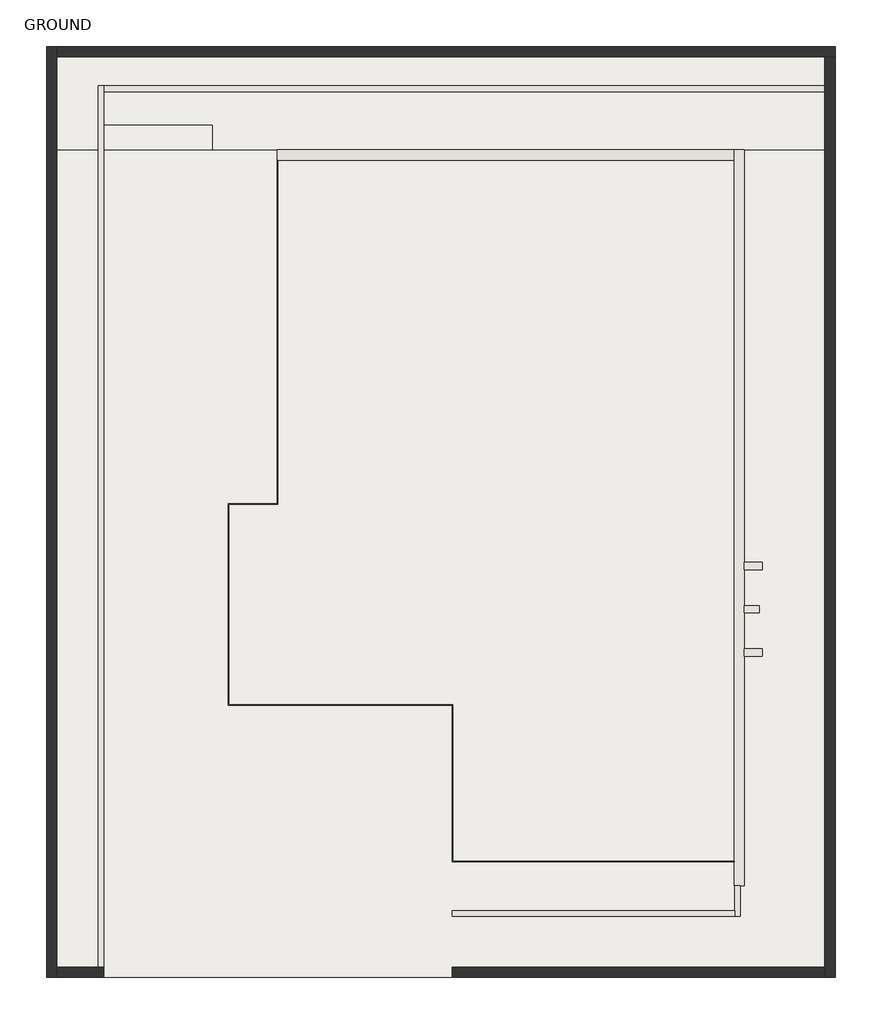
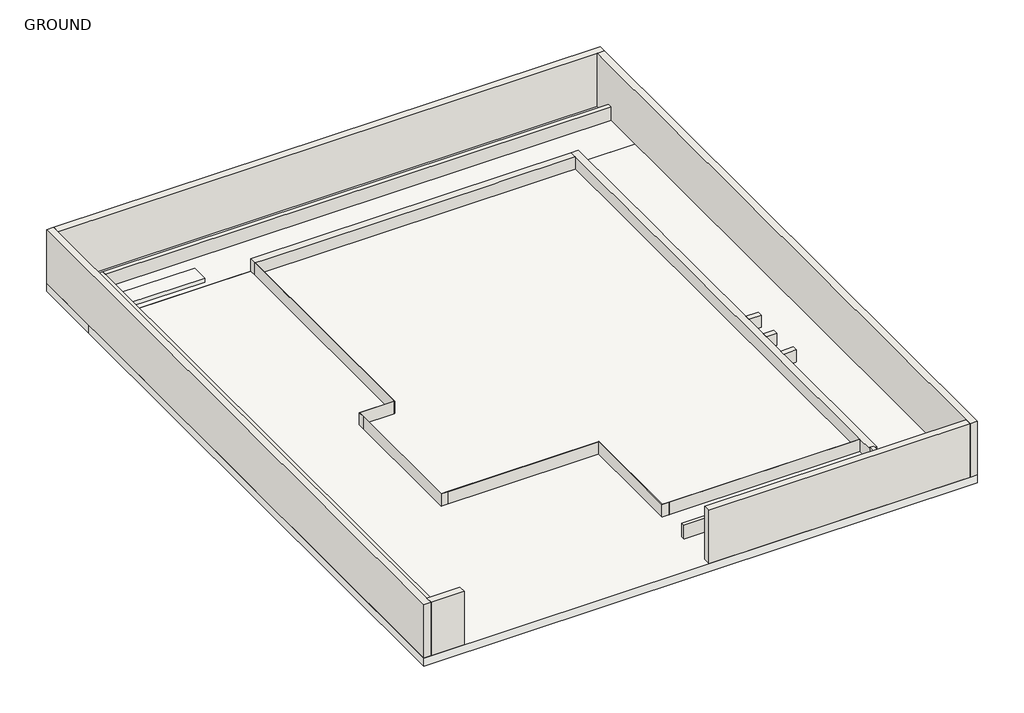
# One storey: 20 walls, 3 slabs.
"""IFC4 building model written with IfcOpenShell, lengths in millimetres."""

from ifc_helpers import new_model, si_unit, frame, origin, origin_with_axes, place, context, project, spatial, polyline, outline, extrude, faceted_brep, element, save

model = new_model("IFC4")

# Units and contexts
model_context = context("Model", 3, world=origin())
ifc_project = project(units=[si_unit("LENGTHUNIT", "METRE", prefix="MILLI")], contexts=[model_context])

# Site, building, storey
site = spatial("IfcSite", under=ifc_project)
building = spatial("IfcBuilding", under=site)
storey = spatial("IfcBuildingStorey", under=building, Name="GROUND", Elevation=0.0)

# Slabs
placement = place(None, origin())
element("IfcSlab", 1, ObjectType="6\" 3", at=placement, inside=storey, context=model_context, shape_type="SweptSolid", body=[
    extrude(outline(polyline([(-6900.6561363, 9478.9935985), (-9643.8561363, 9478.9935985), (-9643.8561363, 10088.5935985), (-6900.6561363, 10088.5935985), (-6900.6561363, 9478.9935985)])), frame((0.0, 0.0, 152.4), z_axis=(0.0, 0.0, 1.0), x_axis=(1.0, 0.0, 0.0)), (0.0, 0.0, 1.0), 152.4),
])
element("IfcSlab", 2, ObjectType="Generic - 12\"", at=placement, inside=storey, context=model_context, shape_type="SweptSolid", body=[
    extrude(outline(polyline([(8479.5731195, 9466.0221373), (8479.5731195, -10955.3064015), (-10990.0561363, -10955.3064015), (-10990.0561363, 9466.0221373), (8479.5731195, 9466.0221373)])), frame((0.0, 0.0, -304.8), z_axis=(0.0, 0.0, 1.0), x_axis=(1.0, 0.0, 0.0)), (0.0, 0.0, 1.0), 304.8),
])
element("IfcSlab", 3, ObjectType="Generic - 12\" 2", at=placement, inside=storey, context=model_context, shape_type="SweptSolid", body=[
    extrude(outline(polyline([(8479.5731195, 12031.6935985), (8479.5731195, 9466.0221373), (-10990.0561363, 9466.0221373), (-10990.0561363, 12031.6935985), (8479.5731195, 12031.6935985)])), frame((0.0, 0.0, -304.8), z_axis=(0.0, 0.0, 1.0), x_axis=(1.0, 0.0, 0.0)), (0.0, 0.0, 1.0), 304.8),
])

# Walls
element("IfcWall", 4, ObjectType="4.5\"", at=placement, inside=storey, context=model_context, shape_type="Brep", body=[
    faceted_brep([(-9574.0061363, -10701.3064015, 0.0), (-9574.0061363, 10920.4435985, 0.0), (-9574.0061363, 11060.1435985, 0.0), (-9574.0061363, 11060.1435985, 508.0), (-9574.0061363, 10920.4435985, 508.0), (-9574.0061363, -10701.3064015, 508.0), (-9713.7061363, -10701.3064015, 0.0), (-9713.7061363, -10701.3064015, 508.0), (-9713.7061363, 11060.1435985, 508.0), (-9713.7061363, 11060.1435985, 0.0)], [[[0, 1, 2, 3, 4, 5]], [[6, 7, 8, 9]], [[2, 1, 0, 6, 9]], [[5, 4, 3, 8, 7]], [[3, 2, 9, 8]], [[0, 5, 7, 6]]]),
])
element("IfcWall", 5, ObjectType="4.5\"", at=placement, inside=storey, context=model_context, shape_type="SweptSolid", body=[
    extrude(outline(polyline([(8225.5731195, 10920.4435985), (-9574.0061363, 10920.4435985), (-9574.0061363, 11060.1435985), (8225.5731195, 11060.1435985), (8225.5731195, 10920.4435985)])), origin_with_axes(), (0.0, 0.0, 1.0), 508.0),
])
element("IfcWall", 6, ObjectType="4.5\"", at=placement, inside=storey, context=model_context, shape_type="Brep", body=[
    faceted_brep([(6002.8084916, -8694.7064015, 508.0), (6002.8084916, -8694.7064015, 0.0), (6002.8084916, -9304.3064015, 0.0), (6002.8084916, -9444.0064015, 0.0), (6002.8084916, -9444.0064015, 508.0), (6002.8084916, -9304.3064015, 508.0), (6142.5084916, -8694.7064015, 0.0), (6142.5084916, -8694.7064015, 508.0), (6142.5084916, -9444.0064015, 508.0), (6142.5084916, -9444.0064015, 0.0)], [[[0, 1, 2, 3, 4, 5]], [[6, 7, 8, 9]], [[3, 2, 1, 6, 9]], [[0, 5, 4, 8, 7]], [[4, 3, 9, 8]], [[0, 7, 6, 1]]]),
])
element("IfcWall", 7, ObjectType="4.5\"", at=placement, inside=storey, context=model_context, shape_type="SweptSolid", body=[
    extrude(outline(polyline([(-969.7561363, -9304.3064015), (6002.8084916, -9304.3064015), (6002.8084916, -9444.0064015), (-969.7561363, -9444.0064015), (-969.7561363, -9304.3064015)])), origin_with_axes(), (0.0, 0.0, 1.0), 508.0),
])
element("IfcWall", 8, ObjectType="6\" WALL", at=placement, inside=storey, context=model_context, shape_type="SweptSolid", body=[
    extrude(outline(polyline([(6688.3438637, -885.2318739), (6244.1084916, -885.2318739), (6244.1084916, -707.4318739), (6688.3438637, -707.4318739), (6688.3438637, -885.2318739)])), origin_with_axes(), (0.0, 0.0, 1.0), 457.2),
])
element("IfcWall", 9, ObjectType="6\" WALL", at=placement, inside=storey, context=model_context, shape_type="SweptSolid", body=[
    extrude(outline(polyline([(6244.1084916, -2840.9358398), (6688.3438637, -2840.9358398), (6688.3438637, -3018.7358398), (6244.1084916, -3018.7358398), (6244.1084916, -2840.9358398)])), origin_with_axes(), (0.0, 0.0, 1.0), 457.2),
])
element("IfcWall", 10, ObjectType="6\" WALL", at=placement, inside=storey, context=model_context, shape_type="SweptSolid", body=[
    extrude(outline(polyline([(6244.1084916, -1774.2318739), (6612.1438637, -1774.2318739), (6612.1438637, -1952.0318739), (6244.1084916, -1952.0318739), (6244.1084916, -1774.2318739)])), origin_with_axes(), (0.0, 0.0, 1.0), 457.2),
])
element("IfcWall", 11, ObjectType="9\"", at=placement, inside=storey, context=model_context, shape_type="SweptSolid", body=[
    extrude(outline(polyline([(5990.1084916, -8097.8064015), (-715.7561363, -8097.8064015), (-715.7561363, -8085.3778627), (5990.1084916, -8085.3778627), (5990.1084916, -8097.8064015)])), origin_with_axes(), (0.0, 0.0, 1.0), 457.2),
])
element("IfcWall", 12, ObjectType="9\"", at=placement, inside=storey, context=model_context, shape_type="Brep", body=[
    faceted_brep([(5990.1084916, 9478.9935985, 0.0), (5990.1084916, 9224.9935985, 0.0), (5990.1084916, -8085.3778627, 0.0), (5990.1084916, -8097.8064015, 0.0), (5990.1084916, -8694.7064015, 0.0), (5990.1084916, -8694.7064015, 457.2), (5990.1084916, -8097.8064015, 457.2), (5990.1084916, -8085.3778627, 457.2), (5990.1084916, 1978.0935985, 457.2), (5990.1084916, 2943.2935985, 457.2), (5990.1084916, 3938.6935985, 457.2), (5990.1084916, 4751.4935985, 457.2), (5990.1084916, 9224.9935985, 457.2), (5990.1084916, 9478.9935985, 457.2), (6244.1084916, 9478.9935985, 0.0), (6244.1084916, 9478.9935985, 457.2), (6244.1084916, 4751.4935985, 457.2), (6244.1084916, 3938.6935985, 457.2), (6244.1084916, 2943.2935985, 457.2), (6244.1084916, 1978.0935985, 457.2), (6244.1084916, -707.4318739, 457.2), (6244.1084916, -885.2318739, 457.2), (6244.1084916, -1774.2318739, 457.2), (6244.1084916, -1952.0318739, 457.2), (6244.1084916, -2840.9358398, 457.2), (6244.1084916, -3018.7358398, 457.2), (6244.1084916, -8694.7064015, 457.2), (6244.1084916, -8694.7064015, 0.0), (6244.1084916, -3018.7358398, 0.0), (6244.1084916, -2840.9358398, 0.0), (6244.1084916, -1952.0318739, 0.0), (6244.1084916, -1774.2318739, 0.0), (6244.1084916, -885.2318739, 0.0), (6244.1084916, -707.4318739, 0.0), (6142.5084916, -8694.7064015, 0.0), (6002.8084916, -8694.7064015, 0.0)], [[[0, 1, 2, 3, 4, 5, 6, 7, 8, 9, 10, 11, 12, 13]], [[14, 15, 16, 17, 18, 19, 20, 21, 22, 23, 24, 25, 26, 27, 28, 29, 30, 31, 32, 33]], [[4, 3, 2, 1, 0, 14, 33, 32, 31, 30, 29, 28, 27, 34, 35]], [[5, 4, 35, 34, 27, 26]], [[13, 12, 11, 10, 9, 8, 7, 6, 5, 26, 25, 24, 23, 22, 21, 20, 19, 18, 17, 16, 15]], [[0, 13, 15, 14]]]),
])
element("IfcWall", 13, ObjectType="9\"", at=placement, inside=storey, context=model_context, shape_type="Brep", body=[
    faceted_brep([(5990.1084916, 9478.9935985, 0.0), (-5287.7561363, 9478.9935985, 0.0), (-5287.7561363, 9478.9935985, 457.2), (5990.1084916, 9478.9935985, 457.2), (5990.1084916, 9224.9935985, 0.0), (5990.1084916, 9224.9935985, 457.2), (3322.8438637, 9224.9935985, 457.2), (3145.0438637, 9224.9935985, 457.2), (-5033.7561363, 9224.9935985, 457.2), (-5287.7561363, 9224.9935985, 457.2), (-5287.7561363, 9224.9935985, 0.0), (-5033.7561363, 9224.9935985, 0.0), (3145.0438637, 9224.9935985, 0.0), (3322.8438637, 9224.9935985, 0.0)], [[[0, 1, 2, 3]], [[4, 5, 6, 7, 8, 9, 10, 11, 12, 13]], [[1, 0, 4, 13, 12, 11, 10]], [[3, 2, 9, 8, 7, 6, 5]], [[0, 3, 5, 4]], [[2, 1, 10, 9]]]),
])
element("IfcWall", 14, ObjectType="9\"", at=placement, inside=storey, context=model_context, shape_type="Brep", body=[
    faceted_brep([(-5287.7561363, 9224.9935985, 457.2), (-5287.7561363, 9224.9935985, 0.0), (-5287.7561363, 741.1221373, 0.0), (-5287.7561363, 728.4221373, 0.0), (-5287.7561363, 728.4221373, 457.2), (-5287.7561363, 741.1221373, 457.2), (-5275.0561363, 9224.9935985, 0.0), (-5275.0561363, 728.4221373, 0.0), (-5275.0561363, 728.4221373, 457.2), (-5275.0561363, 9224.9935985, 457.2)], [[[0, 1, 2, 3, 4, 5]], [[3, 2, 1, 6, 7]], [[0, 5, 4, 8, 9]], [[1, 0, 9, 6]], [[7, 8, 4, 3]], [[8, 7, 6, 9]]]),
])
element("IfcWall", 15, ObjectType="9\"", at=placement, inside=storey, context=model_context, shape_type="SweptSolid", body=[
    extrude(outline(polyline([(-6507.1004467, 741.1221373), (-5287.7561363, 741.1221373), (-5287.7561363, 728.4221373), (-6494.2561363, 728.4221373), (-6494.2561363, 487.1221373), (-6507.1004467, 487.1221373), (-6507.1004467, 741.1221373)])), origin_with_axes(), (0.0, 0.0, 1.0), 457.2),
])
element("IfcWall", 16, ObjectType="9\"", at=placement, inside=storey, context=model_context, shape_type="SweptSolid", body=[
    extrude(outline(polyline([(-6507.1004467, -4237.1266767), (-6507.1004467, 487.1221373), (-6494.2561363, 487.1221373), (-6494.2561363, -4224.5778627), (-6253.1004467, -4224.5778627), (-6253.1004467, -4237.1266767), (-6507.1004467, -4237.1266767)])), origin_with_axes(), (0.0, 0.0, 1.0), 457.2),
])
element("IfcWall", 17, ObjectType="9\"", at=placement, inside=storey, context=model_context, shape_type="SweptSolid", body=[
    extrude(outline(polyline([(-969.7561363, -4237.1266767), (-6253.1004467, -4237.1266767), (-6253.1004467, -4224.5778627), (-969.7561363, -4224.5778627), (-969.7561363, -4237.1266767)])), origin_with_axes(), (0.0, 0.0, 1.0), 457.2),
])
element("IfcWall", 18, ObjectType="9\"", at=placement, inside=storey, context=model_context, shape_type="Brep", body=[
    faceted_brep([(-715.7561363, -8097.8064015, 457.2), (-715.7561363, -8097.8064015, 0.0), (-715.7561363, -8085.3778627, 0.0), (-715.7561363, -8085.3778627, 457.2), (-969.7561363, -8097.8064015, 0.0), (-969.7561363, -8097.8064015, 457.2), (-969.7561363, -4237.1266767, 457.2), (-969.7561363, -4224.5778627, 457.2), (-969.7561363, -4224.5778627, 0.0), (-969.7561363, -4237.1266767, 0.0), (-957.0561363, -4224.5778627, 0.0), (-957.0561363, -8085.3778627, 0.0), (-957.0561363, -8085.3778627, 457.2), (-957.0561363, -4224.5778627, 457.2)], [[[0, 1, 2, 3]], [[4, 5, 6, 7, 8, 9]], [[1, 4, 9, 8, 10, 11, 2]], [[5, 0, 3, 12, 13, 7, 6]], [[1, 0, 5, 4]], [[11, 12, 3, 2]], [[12, 11, 10, 13]], [[13, 10, 8, 7]]]),
])
element("IfcWall", 19, ObjectType="9\"", at=placement, inside=storey, context=model_context, shape_type="Brep", body=[
    faceted_brep([(-10736.0561363, -10955.3064015, 0.0), (-10736.0561363, -10701.3064015, 0.0), (-10736.0561363, 11777.6935985, 0.0), (-10736.0561363, 12031.6935985, 0.0), (-10736.0561363, 12031.6935985, 1981.2), (-10736.0561363, 11777.6935985, 1981.2), (-10736.0561363, -10701.3064015, 1981.2), (-10736.0561363, -10955.3064015, 1981.2), (-10990.0561363, -10955.3064015, 0.0), (-10990.0561363, -10955.3064015, 1981.2), (-10990.0561363, 12031.6935985, 1981.2), (-10990.0561363, 12031.6935985, 0.0)], [[[0, 1, 2, 3, 4, 5, 6, 7]], [[8, 9, 10, 11]], [[3, 2, 1, 0, 8, 11]], [[7, 6, 5, 4, 10, 9]], [[4, 3, 11, 10]], [[0, 7, 9, 8]]]),
])
element("IfcWall", 20, ObjectType="9\"", at=placement, inside=storey, context=model_context, shape_type="Brep", body=[
    faceted_brep([(-10736.0561363, 11777.6935985, 0.0), (8225.5731195, 11777.6935985, 0.0), (8479.5731195, 11777.6935985, 0.0), (8479.5731195, 11777.6935985, 1981.2), (8225.5731195, 11777.6935985, 1981.2), (-10736.0561363, 11777.6935985, 1981.2), (-10736.0561363, 12031.6935985, 0.0), (-10736.0561363, 12031.6935985, 1981.2), (8479.5731195, 12031.6935985, 1981.2), (8479.5731195, 12031.6935985, 0.0)], [[[0, 1, 2, 3, 4, 5]], [[6, 7, 8, 9]], [[2, 1, 0, 6, 9]], [[5, 4, 3, 8, 7]], [[0, 5, 7, 6]], [[3, 2, 9, 8]]]),
])
element("IfcWall", 21, ObjectType="9\"", at=placement, inside=storey, context=model_context, shape_type="Brep", body=[
    faceted_brep([(8225.5731195, 11777.6935985, 0.0), (8225.5731195, 11060.1435985, 0.0), (8225.5731195, 10920.4435985, 0.0), (8225.5731195, -10701.3064015, 0.0), (8225.5731195, -10955.3064015, 0.0), (8225.5731195, -10955.3064015, 1981.2), (8225.5731195, -10701.3064015, 1981.2), (8225.5731195, 11777.6935985, 1981.2), (8479.5731195, 11777.6935985, 0.0), (8479.5731195, 11777.6935985, 1981.2), (8479.5731195, -10955.3064015, 1981.2), (8479.5731195, -10955.3064015, 0.0)], [[[0, 1, 2, 3, 4, 5, 6, 7]], [[8, 9, 10, 11]], [[4, 3, 2, 1, 0, 8, 11]], [[7, 6, 5, 10, 9]], [[0, 7, 9, 8]], [[5, 4, 11, 10]]]),
])
element("IfcWall", 22, ObjectType="9\"", at=placement, inside=storey, context=model_context, shape_type="SweptSolid", body=[
    extrude(outline(polyline([(-969.7561363, -10701.3064015), (8225.5731195, -10701.3064015), (8225.5731195, -10955.3064015), (-969.7561363, -10955.3064015), (-969.7561363, -10701.3064015)])), origin_with_axes(), (0.0, 0.0, 1.0), 1981.2),
])
element("IfcWall", 23, ObjectType="9\"", at=placement, inside=storey, context=model_context, shape_type="Brep", body=[
    faceted_brep([(-10736.0561363, -10955.3064015, 0.0), (-9574.0061363, -10955.3064015, 0.0), (-9574.0061363, -10955.3064015, 1981.2), (-10736.0561363, -10955.3064015, 1981.2), (-10736.0561363, -10701.3064015, 0.0), (-10736.0561363, -10701.3064015, 1981.2), (-9574.0061363, -10701.3064015, 1981.2), (-9574.0061363, -10701.3064015, 508.0), (-9574.0061363, -10701.3064015, 0.0), (-9713.7061363, -10701.3064015, 0.0)], [[[0, 1, 2, 3]], [[4, 5, 6, 7, 8, 9]], [[1, 0, 4, 9, 8]], [[3, 2, 6, 5]], [[0, 3, 5, 4]], [[2, 1, 8, 7, 6]]]),
])

save(model, "model.ifc")

# Revit data of these elements
# Type "6\" 3"
#   Assembly Code = "B1010"
#   Function = 0
#   Layers, outside or top first: 0' - 6" "Concrete, Cast-in-Place gray" (function 1)
# Type "Generic - 12\""
#   Assembly Code = "B1010"
#   Function = 0
#   Layers, outside or top first: 1' - 0" no material (function 1)
# Type "Generic - 12\" 2"
#   Assembly Code = "B1010"
#   Function = 0
#   Layers, outside or top first: 1' - 0" "Grass" (function 1)
# Type "4.5\""
#   Assembly Code = "B2010"
#   Layers, outside or top first: 0' - 0 1/2" no material (function 4); 0' - 4 1/2" "Acoustic Ceiling Tile 24 x 24" (function 1); 0' - 0 1/2" no material (function 4)
# Type "6\" WALL"
#   Assembly Code = "B2010"
#   Layers, outside or top first: 0' - 0 1/2" no material (function 4); 0' - 6" no material (function 1); 0' - 0 1/2" no material (function 4)
# Type "9\""
#   Assembly Code = "B2010"
#   Layers, outside or top first: 0' - 0 1/2" no material (function 4); 0' - 9" no material (function 1); 0' - 0 1/2" no material (function 4)
# Element 1 (IfcSlab, "6\" 3")
#   Height Offset From Level = 1' - 0"
#   built-in parameter 1001954 = 1
#   Phase Created = New Construction
#   Materials on its faces: "Concrete, Cast-in-Place gray"
# Element 2 (IfcSlab, "Generic - 12\"")
#   Height Offset From Level = 0' - 0"
#   built-in parameter 1001954 = 1
#   Phase Created = New Construction
#   Materials on its faces: "Default Floor", "black"
# Element 3 (IfcSlab, "Generic - 12\" 2")
#   Height Offset From Level = 0' - 0"
#   built-in parameter 1001954 = 1
#   Phase Created = New Construction
#   Materials on its faces: "Grass", "black"
# Elements 4, 5, 6, 7 (IfcWall, "4.5\"")
#   Top Offset = 0' - 2"
#   Base Offset = 0' - 0"
#   wall height = 1' - 8"
#   Phase Created = New Construction
#   Base Constraint = GROUND
#   Top Constraint = GROUND FLOOR
#   Materials on its faces: "WHITE", "Default Wall"
# Elements 8, 9, 10 (IfcWall, "6\" WALL")
#   Top Offset = 0' - 0"
#   Base Offset = 0' - 0"
#   wall height = 1' - 6"
#   Phase Created = New Construction
#   Base Constraint = GROUND
#   Top Constraint = GROUND FLOOR
#   Materials on its faces: "Default Wall"
# Elements 11, 12, 13, 14, 15, 16, 17, 18 (IfcWall, "9\"")
#   Top Offset = 0' - 0"
#   Base Offset = 0' - 0"
#   wall height = 1' - 6"
#   Phase Created = New Construction
#   Base Constraint = GROUND
#   Top Constraint = GROUND FLOOR
#   Materials on its faces: "Default Wall"
# Element 19 (IfcWall, "9\"")
#   Top Offset = 5' - 0"
#   Base Offset = 0' - 0"
#   wall height = 6' - 6"
#   Phase Created = New Construction
#   Base Constraint = GROUND
#   Top Constraint = GROUND FLOOR
#   Materials on its faces: "black", "Default Wall"
# Elements 20, 21, 22 (IfcWall, "9\"")
#   Top Offset = 5' - 0"
#   Base Offset = 0' - 0"
#   wall height = 6' - 6"
#   Phase Created = New Construction
#   Base Constraint = GROUND
#   Top Constraint = GROUND FLOOR
#   Materials on its faces: "Default Wall", "black"
# Element 23 (IfcWall, "9\"")
#   Top Offset = 5' - 0"
#   Base Offset = 0' - 0"
#   wall height = 6' - 6"
#   Phase Created = New Construction
#   Base Constraint = GROUND
#   Top Constraint = GROUND FLOOR
#   Materials on its faces: "black", "Default Wall", "WHITE"
# Materials
#   "Concrete, Cast-in-Place gray": class "Concrete", colour RGB 192 192 192, transparency 0, Description = "Cast-in-place concrete", Cost = 0
#   "Grass": class "Generic", colour RGB 104 137 66, transparency 0, Description = "Physical material.", Cost = 0
#   "Acoustic Ceiling Tile 24 x 24": class "Generic", colour RGB 232 232 232, transparency 0, Description = "Acoustic Ceiling Tile 24 x 24", Cost = 0
#   "Default Floor": colour RGB 128 128 128, transparency 0, Cost = 0
#   "black": class "Generic", colour RGB 120 120 120, transparency 0, Cost = 0
#   "WHITE": class "Generic", colour RGB 120 120 120, transparency 0, Cost = 0
#   "Default Wall": colour RGB 128 128 128, transparency 0, Cost = 0
